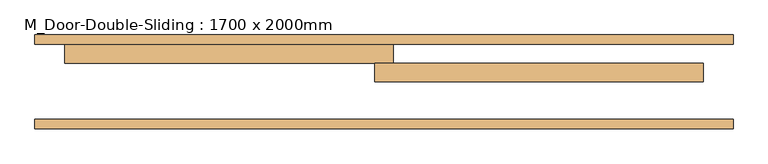
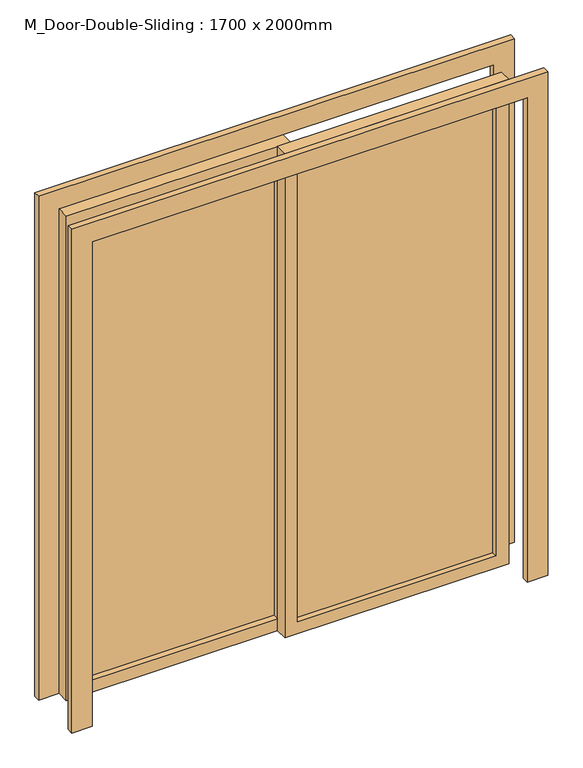
"""IFC4 building model written with IfcOpenShell, lengths in millimetres: door geometry, M_Door-Double-Sliding : 1700 x 2000mm."""

from ifc_helpers import new_model, si_unit, frame, origin, place, context, project, spatial, polyline, outline, extrude, source, transform, mapped, element, save


def m_door_double_sliding_1700_x_2000mm_9ea34811(model_context):
    return source(origin(), model_context, "Body", "SweptSolid", [
        extrude(outline(polyline([(0.0, -930.0), (0.0, -850.0), (2000.0, -850.0), (2000.0, 850.0), (0.0, 850.0), (0.0, 930.0), (2080.0, 930.0), (2080.0, -930.0), (0.0, -930.0)])), frame((0.0, 2.0, 0.0), z_axis=(0.0, 1.0, 0.0), x_axis=(0.0, 0.0, 1.0)), (0.0, 0.0, 1.0), 25.0),
        extrude(outline(polyline([(0.0, 930.0), (2080.0, 930.0), (2080.0, -930.0), (0.0, -930.0), (0.0, -850.0), (2000.0, -850.0), (2000.0, 850.0), (0.0, 850.0), (0.0, 930.0)])), frame((0.0, 227.0, 0.0), z_axis=(0.0, 1.0, 0.0), x_axis=(0.0, 0.0, 1.0)), (0.0, 0.0, 1.0), 25.0),
        extrude(outline(polyline([(2000.0, -25.0), (0.0, -25.0), (0.0, 850.0), (2000.0, 850.0), (2000.0, -25.0)]), holes=[polyline([(1950.0, 25.0), (1950.0, 800.0), (50.0, 800.0), (50.0, 25.0), (1950.0, 25.0)])]), frame((0.0, 127.0, 0.0), z_axis=(0.0, 1.0, 0.0), x_axis=(0.0, 0.0, 1.0)), (0.0, 0.0, 1.0), 50.0),
        extrude(outline(polyline([(2000.0, 25.0), (2000.0, -850.0), (0.0, -850.0), (0.0, 25.0), (2000.0, 25.0)]), holes=[polyline([(1950.0, -25.0), (50.0, -25.0), (50.0, -800.0), (1950.0, -800.0), (1950.0, -25.0)])]), frame((0.0, 177.0, 0.0), z_axis=(0.0, 1.0, 0.0), x_axis=(0.0, 0.0, 1.0)), (0.0, 0.0, 1.0), 50.0),
        extrude(outline(polyline([(25.0, 155.175), (800.0, 155.175), (800.0, 148.825), (25.0, 148.825), (25.0, 155.175)])), frame((0.0, 0.0, 50.0), z_axis=(0.0, 0.0, 1.0), x_axis=(1.0, 0.0, 0.0)), (0.0, 0.0, 1.0), 1900.0),
        extrude(outline(polyline([(-25.0, 200.025), (-800.0, 200.025), (-800.0, 206.375), (-25.0, 206.375), (-25.0, 200.025)])), frame((0.0, 0.0, 50.0), z_axis=(0.0, 0.0, 1.0), x_axis=(1.0, 0.0, 0.0)), (0.0, 0.0, 1.0), 1900.0),
    ])


if __name__ == "__main__":
    model = new_model("IFC4")
    model_context = context("Model", 3, world=origin())
    ifc_project = project(units=[si_unit("LENGTHUNIT", "METRE", prefix="MILLI")], contexts=[model_context])
    site = spatial("IfcSite", under=ifc_project)
    building = spatial("IfcBuilding", under=site)
    placement = place(None, origin())
    m_door_double_sliding_1700_x_2000mm_shape = m_door_double_sliding_1700_x_2000mm_9ea34811(model_context)
    element("IfcDoor", 1, ObjectType="M_Door-Double-Sliding : 1700 x 2000mm", at=placement, inside=building, context=model_context, shape_type="MappedRepresentation", body=[
        mapped(m_door_double_sliding_1700_x_2000mm_shape, transform((0.0, 0.0, 0.0), x_axis=(1.0, 0.0, 0.0), y_axis=(0.0, 1.0, 0.0), z_axis=(0.0, 0.0, 1.0))),
    ])
    save(model, "model.ifc")

# Revit data of these elements
# Type "M_Door-Double-Sliding : 1700 x 2000mm"
#   Type Mark = "22"
#   Construction Type Id = "opn-d45"
#   Assembly Code = "C1020"
#   Analytic Construction = "Wood frame, double glass door "
#   Thickness = 0' - 1.9685"
#   Thermal Resistance (R) = 0.31964 (m²·K)/W
#   Heat Transfer Coefficient (U) = 3.12872 W/(m²·K)
#   Height = 6' - 6.74016"
#   Rail Width = 0' - 1.9685"
#   Stiles = 0' - 1.9685"
#   Trim Projection Ext = 0' - 0.98425"
#   Trim Projection Int = 0' - 0.98425"
#   Trim Width = 0' - 3.14961"
#   Width = 5' - 6.92913"
#   Define Thermal Properties by = 1
#   Glazing = Glass
#   Panel Material = Wood - Birch - Solid Stained Light Low Gloss
#   Trim Material = Paint - Sienna
#   Visual Light Transmittance = 0
#   Solar Heat Gain Coefficient = 0
#   Function = (empty or 0)
#   Wall Closure = (empty or 0)
# Element 1 (IfcDoor, "M_Door-Double-Sliding : 1700 x 2000mm")
#   Materials on its faces: "Paint - Sienna", "Wood - Birch - Solid Stained Light Low Gloss", "Glass"
# Materials
#   "Glass": class "Glass", colour RGB 218 227 224, transparency 0.85, Description = "Soda Lime Glass", Cost = 0
#   "Wood - Birch - Solid Stained Light Low Gloss": class "Wood", colour RGB 210 159 95, transparency 0, Cost = 0
#   "Paint - Sienna": colour RGB 118 70 51, transparency 0, Cost = 0
